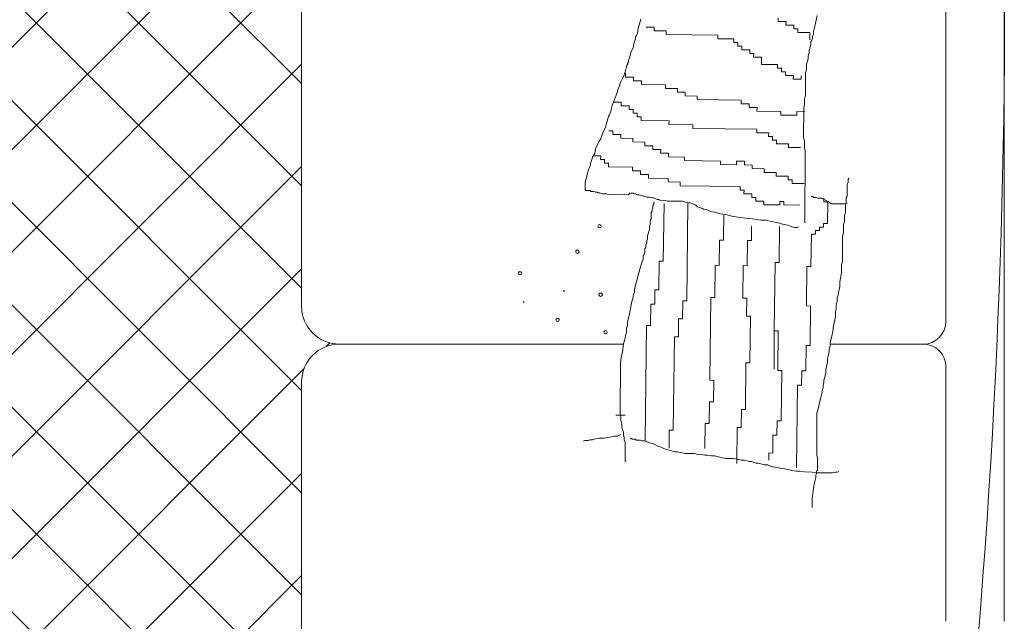
# Model space of a CAD drawing. Units: inches. Extents: x -466983 to 1020, y 324 to 318697.
# Tile 89 of 97: x 776 to 810, y 900 to 921. Entities that reach past the tile are written whole.
import ezdxf

# ---------------------------------------------------------------- set-up
doc = ezdxf.new("R2010")
doc.units = ezdxf.units.IN
doc.header["$MEASUREMENT"] = 0
doc.layers.add('A-FLOR-PATT', color=252, linetype='Continuous', lineweight=13)
doc.layers.add('A-FURN', color=8, linetype='Continuous', lineweight=18)

# ---------------------------------------------------------------- blocks, each defined once
blk = doc.blocks.new('L Shaped Sofa')
at = {"ltscale": 2}
for p, q in [((2356.696, 767.567), (2377.232, 767.567)), ((2377.232, 767.567), (2392.324, 767.567)), ((2429.959, 767.567), (2397.1, 767.567)), ((2394.712, 747.255), (2394.712, 765.179)), ((2388.636, 749.7), (2388.588, 749.809)), ((2388.634, 749.483), (2388.636, 749.7)), ((2388.683, 749.374), (2388.634, 749.483)), ((2388.682, 749.212), (2388.683, 749.374)), ((2404.345, 749.138), (2404.346, 749.301)), ((2404.346, 749.301), (2404.395, 749.355)), ((2404.395, 749.355), (2404.397, 749.626)), ((2404.397, 749.626), (2404.446, 749.68)), ((2404.446, 749.68), (2404.934, 749.678)), ((2404.934, 749.678), (2405.713, 749.457)), ((2405.713, 749.457), (2406.005, 749.347)), ((2406.005, 749.347), (2406.103, 749.347)), ((2406.103, 749.347), (2406.541, 749.182)), ((2388.729, 749.049), (2388.682, 749.212)), ((2388.776, 748.778), (2388.729, 749.049)), ((2388.775, 748.507), (2388.776, 748.778)), ((2404.193, 748.326), (2404.195, 748.597)), ((2404.195, 748.597), (2404.245, 748.759)), ((2404.245, 748.759), (2404.246, 748.868)), ((2404.246, 748.868), (2404.295, 748.922)), ((2404.295, 749.03), (2404.345, 749.138)), ((2404.295, 748.922), (2404.295, 749.03)), ((2406.349, 748.446), (2406.352, 748.698)), ((2406.352, 748.698), (2406.579, 748.695)), ((2406.541, 749.182), (2406.735, 749.073)), ((2406.579, 748.695), (2406.585, 749.199)), ((2406.735, 749.073), (2407.028, 749.017)), ((2407.028, 749.017), (2407.514, 748.798)), ((2407.514, 748.798), (2407.66, 748.689)), ((2407.66, 748.689), (2407.806, 748.634)), ((2407.806, 748.634), (2408.001, 748.579)), ((2388.822, 748.235), (2388.775, 748.507)), ((2388.917, 747.801), (2388.822, 748.235)), ((2404.136, 746.971), (2404.144, 748.218)), ((2404.144, 748.218), (2404.193, 748.326)), ((2405.873, 746.688), (2405.892, 748.199)), ((2405.892, 748.199), (2406.119, 748.197)), ((2406.119, 748.197), (2406.122, 748.449)), ((2406.122, 748.449), (2406.349, 748.446)), ((2408.001, 748.579), (2408.147, 748.524)), ((2408.147, 748.524), (2408.342, 748.415)), ((2408.157, 747.92), (2408.16, 748.172)), ((2408.342, 748.415), (2408.926, 748.249)), ((2408.926, 748.249), (2409.072, 748.194)), ((2409.072, 748.194), (2409.17, 748.14)), ((2409.17, 748.14), (2409.316, 748.085)), ((2409.316, 748.085), (2409.51, 748.03)), ((2409.51, 748.03), (2409.754, 747.974)), ((2409.754, 747.974), (2410.63, 747.645)), ((2388.916, 747.638), (2388.917, 747.801)), ((2389.012, 747.421), (2388.916, 747.638)), ((2389.304, 747.311), (2389.5, 747.365)), ((2389.5, 747.365), (2389.695, 747.364)), ((2389.695, 747.364), (2389.89, 747.417)), ((2389.89, 747.417), (2390.086, 747.416)), ((2390.086, 747.416), (2390.33, 747.469)), ((2390.234, 747.741), (2390.23, 747.144)), ((2390.33, 747.469), (2393.55, 747.454)), ((2393.55, 747.454), (2393.843, 747.398)), ((2393.843, 747.398), (2394.33, 747.288)), ((2407.688, 746.666), (2407.697, 747.422)), ((2407.697, 747.422), (2407.924, 747.419)), ((2407.924, 747.419), (2407.93, 747.923)), ((2407.93, 747.923), (2408.157, 747.92)), ((2409.733, 746.893), (2409.739, 747.397)), ((2409.739, 747.397), (2409.966, 747.394)), ((2409.966, 747.394), (2409.972, 747.898)), ((2410.63, 747.645), (2410.825, 747.59)), ((2410.825, 747.59), (2411.02, 747.48)), ((2411.02, 747.48), (2411.117, 747.48)), ((2411.117, 747.48), (2411.263, 747.425)), ((2411.263, 747.425), (2411.458, 747.316)), ((2387.302, 747.104), (2387.351, 747.158)), ((2387.351, 747.158), (2388.523, 747.152)), ((2388.523, 747.152), (2388.669, 747.206)), ((2388.669, 747.206), (2388.816, 747.205)), ((2388.715, 746.718), (2388.764, 746.772)), ((2388.764, 746.772), (2388.765, 746.826)), ((2388.816, 747.205), (2388.962, 747.259)), ((2388.962, 747.259), (2389.158, 747.258)), ((2389.158, 747.258), (2389.304, 747.311)), ((2394.33, 747.288), (2394.574, 747.287)), ((2394.574, 747.287), (2394.818, 747.231)), ((2394.818, 747.231), (2395.013, 747.176)), ((2395.013, 747.176), (2395.256, 747.121)), ((2395.256, 747.121), (2395.451, 747.066)), ((2395.451, 747.066), (2395.695, 747.064)), ((2395.695, 747.064), (2395.89, 747.009)), ((2395.89, 747.009), (2396.085, 747.008)), ((2396.085, 747.008), (2396.28, 746.953)), ((2396.28, 746.953), (2396.524, 746.898)), ((2396.524, 746.898), (2397.401, 746.731)), ((2397.401, 746.731), (2397.596, 746.676)), ((2404.233, 746.862), (2404.136, 746.971)), ((2404.232, 746.645), (2404.233, 746.862)), ((2409.503, 746.644), (2409.506, 746.896)), ((2409.506, 746.896), (2409.733, 746.893)), ((2411.458, 747.316), (2411.701, 747.206)), ((2411.544, 746.619), (2411.55, 747.123)), ((2411.55, 747.123), (2411.777, 747.12)), ((2411.701, 747.206), (2411.896, 747.151)), ((2411.896, 747.151), (2412.14, 747.096)), ((2412.14, 747.096), (2412.286, 747.041)), ((2412.286, 747.041), (2412.383, 746.986)), ((2412.383, 746.986), (2412.481, 746.986)), ((2412.481, 746.986), (2412.529, 746.931)), ((2412.529, 746.931), (2412.627, 746.931)), ((2412.627, 746.931), (2412.773, 746.876)), ((2412.773, 746.876), (2413.162, 746.766)), ((2413.162, 746.766), (2413.406, 746.656)), ((2388.614, 746.068), (2388.663, 746.176)), ((2388.663, 746.176), (2388.665, 746.447)), ((2388.665, 746.447), (2388.714, 746.501)), ((2388.714, 746.501), (2388.715, 746.718)), ((2397.596, 746.676), (2397.839, 746.621)), ((2397.839, 746.621), (2397.985, 746.566)), ((2397.985, 746.566), (2398.181, 746.565)), ((2398.181, 746.565), (2398.57, 746.455)), ((2398.57, 746.455), (2398.814, 746.399)), ((2398.814, 746.399), (2399.204, 746.289)), ((2399.204, 746.289), (2399.447, 746.234)), ((2399.447, 746.234), (2399.593, 746.179)), ((2399.593, 746.179), (2399.788, 746.123)), ((2399.788, 746.123), (2400.08, 746.014)), ((2403.983, 745.779), (2404.132, 746.266)), ((2404.132, 746.266), (2404.133, 746.374)), ((2404.133, 746.374), (2404.182, 746.482)), ((2404.182, 746.482), (2404.183, 746.591)), ((2404.183, 746.591), (2404.232, 746.645)), ((2405.407, 745.686), (2405.414, 746.19)), ((2405.414, 746.19), (2405.64, 746.187)), ((2405.64, 746.187), (2405.647, 746.691)), ((2405.647, 746.691), (2405.873, 746.688)), ((2407.452, 745.913), (2407.461, 746.669)), ((2407.461, 746.669), (2407.688, 746.666)), ((2408.795, 744.385), (2408.816, 746.148)), ((2408.816, 746.148), (2409.043, 746.145)), ((2409.043, 746.145), (2409.046, 746.397)), ((2409.046, 746.397), (2409.273, 746.394)), ((2409.273, 746.394), (2409.276, 746.646)), ((2409.276, 746.646), (2409.503, 746.644)), ((2411.066, 744.609), (2411.084, 746.12)), ((2411.084, 746.12), (2411.311, 746.118)), ((2411.311, 746.118), (2411.317, 746.621)), ((2411.317, 746.621), (2411.544, 746.619)), ((2413.406, 746.656), (2413.649, 746.601)), ((2413.649, 746.601), (2413.844, 746.545)), ((2413.844, 746.545), (2413.99, 746.491)), ((2413.99, 746.491), (2414.088, 746.49)), ((2414.088, 746.49), (2414.185, 746.435)), ((2414.185, 746.435), (2414.331, 746.381)), ((2414.331, 746.381), (2414.624, 746.325)), ((2414.624, 746.325), (2415.208, 746.16)), ((2388.414, 745.364), (2388.514, 745.688)), ((2388.514, 745.688), (2388.563, 745.797)), ((2388.563, 745.797), (2388.613, 745.959)), ((2388.613, 745.959), (2388.614, 746.068)), ((2388.622, 745.891), (2395.88, 745.802)), ((2395.88, 745.802), (2395.877, 745.55)), ((2395.877, 745.55), (2397.238, 745.534)), ((2397.238, 745.534), (2397.235, 745.282)), ((2400.08, 746.014), (2400.276, 746.013)), ((2400.276, 746.013), (2400.373, 745.958)), ((2400.373, 745.958), (2400.519, 745.903)), ((2400.519, 745.903), (2400.714, 745.902)), ((2400.714, 745.902), (2400.811, 745.848)), ((2400.811, 745.848), (2400.958, 745.847)), ((2400.958, 745.847), (2401.104, 745.792)), ((2401.104, 745.792), (2401.25, 745.791)), ((2401.25, 745.791), (2401.347, 745.737)), ((2401.347, 745.737), (2401.543, 745.736)), ((2401.543, 745.736), (2401.932, 745.625)), ((2401.932, 745.625), (2402.127, 745.625)), ((2402.127, 745.625), (2402.273, 745.57)), ((2402.273, 745.57), (2402.517, 745.569)), ((2402.517, 745.569), (2402.615, 745.514)), ((2402.615, 745.514), (2403.005, 745.512)), ((2403.005, 745.512), (2403.102, 745.457)), ((2403.932, 745.453), (2403.982, 745.616)), ((2403.982, 745.616), (2403.983, 745.779)), ((2405.165, 744.429), (2405.181, 745.689)), ((2405.181, 745.689), (2405.407, 745.686)), ((2407.219, 745.412), (2407.225, 745.916)), ((2407.225, 745.916), (2407.452, 745.913)), ((2414.705, 745.32), (2414.711, 745.824)), ((2388.117, 744.66), (2388.216, 744.877)), ((2388.216, 744.877), (2388.266, 745.039)), ((2388.266, 745.039), (2388.414, 745.364)), ((2397.235, 745.282), (2398.143, 745.271)), ((2398.143, 745.271), (2398.139, 745.019)), ((2398.139, 745.019), (2399.954, 744.997)), ((2399.954, 744.997), (2399.951, 744.745)), ((2403.102, 745.457), (2403.2, 745.457)), ((2403.2, 745.457), (2403.297, 745.402)), ((2403.297, 745.402), (2403.444, 745.402)), ((2403.444, 745.402), (2403.541, 745.347)), ((2403.541, 745.347), (2403.687, 745.346)), ((2403.78, 744.587), (2403.782, 744.966)), ((2403.782, 744.966), (2403.832, 745.02)), ((2403.832, 745.129), (2403.931, 745.345)), ((2403.832, 745.02), (2403.832, 745.129)), ((2403.931, 745.345), (2403.932, 745.453)), ((2406.753, 744.41), (2406.759, 744.914)), ((2406.759, 744.914), (2406.986, 744.911)), ((2406.986, 744.911), (2406.992, 745.415)), ((2406.992, 745.415), (2407.219, 745.412)), ((2414.469, 744.567), (2414.478, 745.323)), ((2414.478, 745.323), (2414.705, 745.32)), ((2387.918, 744.011), (2388.117, 744.66)), ((2388.149, 744.385), (2389.284, 744.371)), ((2389.284, 744.371), (2389.281, 744.119)), ((2399.951, 744.745), (2403.58, 744.7)), ((2403.725, 743.557), (2403.731, 744.478)), ((2403.731, 744.478), (2403.78, 744.587)), ((2404.929, 743.676), (2404.938, 744.432)), ((2404.938, 744.432), (2405.165, 744.429)), ((2406.514, 743.405), (2406.526, 744.412)), ((2406.526, 744.412), (2406.753, 744.41)), ((2408.549, 742.876), (2408.568, 744.388)), ((2408.568, 744.388), (2408.795, 744.385)), ((2410.83, 743.856), (2410.839, 744.612)), ((2410.839, 744.612), (2411.066, 744.609)), ((2414.202, 741.295), (2414.242, 744.57)), ((2414.242, 744.57), (2414.469, 744.567)), ((2387.866, 743.523), (2387.867, 743.685)), ((2387.867, 743.685), (2387.917, 743.848)), ((2387.917, 743.848), (2387.918, 744.011)), ((2389.281, 744.119), (2395.178, 744.047)), ((2395.178, 744.047), (2395.175, 743.795)), ((2395.175, 743.795), (2396.309, 743.781)), ((2396.309, 743.781), (2396.306, 743.53)), ((2404.656, 739.9), (2404.702, 743.679)), ((2404.702, 743.679), (2404.929, 743.676)), ((2410.597, 743.355), (2410.603, 743.859)), ((2410.603, 743.859), (2410.83, 743.856)), ((2387.813, 742.764), (2387.816, 743.36)), ((2387.816, 743.36), (2387.866, 743.523)), ((2396.306, 743.53), (2397.44, 743.516)), ((2397.44, 743.516), (2397.437, 743.264)), ((2397.437, 743.264), (2403.562, 743.189)), ((2403.575, 742.907), (2403.624, 743.069)), ((2403.624, 743.069), (2403.625, 743.232)), ((2403.625, 743.232), (2403.725, 743.557)), ((2406.259, 741.14), (2406.287, 743.408)), ((2406.287, 743.408), (2406.514, 743.405)), ((2410.361, 742.602), (2410.37, 743.358)), ((2410.37, 743.358), (2410.597, 743.355)), ((2387.761, 742.331), (2387.763, 742.656)), ((2387.763, 742.656), (2387.813, 742.764)), ((2403.278, 742.312), (2403.328, 742.474)), ((2403.328, 742.474), (2403.378, 742.583)), ((2403.378, 742.583), (2403.476, 742.69)), ((2403.476, 742.69), (2403.575, 742.907)), ((2408.273, 738.848), (2408.322, 742.879)), ((2408.322, 742.879), (2408.549, 742.876)), ((2410.1, 739.834), (2410.134, 742.605)), ((2410.134, 742.605), (2410.361, 742.602)), ((2387.66, 741.735), (2387.71, 741.951)), ((2387.71, 741.951), (2387.711, 742.114)), ((2387.711, 742.114), (2387.761, 742.331)), ((2388.122, 742.118), (2389.71, 742.098)), ((2389.71, 742.098), (2389.706, 741.847)), ((2389.706, 741.847), (2391.067, 741.83)), ((2391.067, 741.83), (2391.064, 741.578)), ((2392.425, 741.561), (2392.429, 741.813)), ((2392.429, 741.813), (2397.646, 741.75)), ((2403.029, 741.5), (2403.08, 741.771)), ((2403.08, 741.771), (2403.179, 741.987)), ((2403.179, 741.987), (2403.229, 742.204)), ((2403.229, 742.204), (2403.278, 742.312)), ((2387.558, 741.084), (2387.659, 741.518)), ((2387.659, 741.518), (2387.66, 741.735)), ((2391.064, 741.578), (2392.425, 741.561)), ((2397.646, 741.75), (2397.643, 741.498)), ((2397.643, 741.498), (2399.684, 741.473)), ((2399.684, 741.473), (2399.681, 741.221)), ((2399.681, 741.221), (2401.269, 741.201)), ((2401.269, 741.201), (2401.266, 740.949)), ((2402.879, 740.796), (2402.93, 741.175)), ((2402.93, 741.175), (2403.029, 741.5)), ((2406.02, 740.135), (2406.033, 741.143)), ((2406.033, 741.143), (2406.259, 741.14)), ((2413.963, 740.29), (2413.975, 741.298)), ((2413.975, 741.298), (2414.202, 741.295)), ((2387.505, 740.326), (2387.508, 740.814)), ((2387.508, 740.814), (2387.558, 741.084)), ((2401.266, 740.949), (2401.72, 740.944)), ((2401.493, 740.947), (2402.854, 740.93)), ((2401.72, 740.944), (2401.493, 740.947)), ((2402.779, 740.417), (2402.879, 740.796)), ((2387.19, 740.114), (2389.458, 740.086)), ((2387.404, 739.838), (2387.454, 740.055)), ((2387.454, 740.055), (2387.505, 740.326)), ((2389.458, 740.086), (2389.455, 739.834)), ((2402.626, 739.387), (2402.728, 740.037)), ((2402.728, 740.037), (2402.779, 740.417)), ((2404.426, 739.651), (2404.429, 739.903)), ((2404.429, 739.903), (2404.656, 739.9)), ((2406.247, 740.133), (2406.02, 740.135)), ((2406.241, 739.629), (2406.247, 740.133)), ((2413.503, 739.792), (2413.506, 740.044)), ((2413.506, 740.044), (2413.733, 740.041)), ((2413.733, 740.041), (2413.736, 740.293)), ((2413.736, 740.293), (2413.963, 740.29)), ((2387.303, 739.296), (2387.403, 739.621)), ((2387.303, 739.188), (2387.303, 739.296)), ((2387.403, 739.621), (2387.404, 739.838)), ((2389.455, 739.834), (2390.589, 739.82)), ((2390.589, 739.82), (2390.586, 739.568)), ((2390.586, 739.568), (2393.535, 739.532)), ((2393.535, 739.532), (2393.532, 739.28)), ((2393.532, 739.28), (2396.481, 739.244)), ((2396.481, 739.244), (2396.484, 739.496)), ((2396.484, 739.496), (2397.618, 739.482)), ((2397.618, 739.482), (2397.621, 739.734)), ((2397.621, 739.734), (2399.663, 739.709)), ((2399.663, 739.709), (2399.66, 739.457)), ((2399.66, 739.457), (2401.247, 739.438)), ((2401.247, 739.438), (2401.244, 739.186)), ((2402.624, 739.116), (2402.626, 739.387)), ((2404.193, 739.15), (2404.199, 739.654)), ((2404.199, 739.654), (2404.426, 739.651)), ((2406.008, 739.128), (2406.014, 739.632)), ((2406.014, 739.632), (2406.241, 739.629)), ((2409.634, 738.832), (2409.64, 739.335)), ((2409.64, 739.335), (2409.867, 739.333)), ((2409.867, 739.333), (2409.873, 739.836)), ((2409.873, 739.836), (2410.1, 739.834)), ((2413.04, 739.042), (2413.043, 739.294)), ((2413.043, 739.294), (2413.27, 739.291)), ((2413.27, 739.291), (2413.276, 739.795)), ((2413.276, 739.795), (2413.503, 739.792)), ((2387.153, 738.592), (2387.202, 738.755)), ((2387.202, 738.755), (2387.203, 738.917)), ((2387.203, 738.917), (2387.253, 739.026)), ((2387.253, 739.026), (2387.303, 739.188)), ((2394.569, 739.178), (2394.569, 739.178)), ((2401.244, 739.186), (2402.152, 739.175)), ((2402.523, 738.574), (2402.624, 739.116)), ((2403.73, 738.4), (2403.736, 738.904)), ((2403.736, 738.904), (2403.963, 738.901)), ((2403.963, 738.901), (2403.966, 739.153)), ((2403.966, 739.153), (2404.193, 739.15)), ((2405.772, 738.375), (2405.781, 739.131)), ((2405.781, 739.131), (2406.008, 739.128)), ((2408.037, 738.095), (2408.046, 738.851)), ((2408.046, 738.851), (2408.273, 738.848)), ((2409.389, 737.323), (2409.407, 738.834)), ((2409.407, 738.834), (2409.634, 738.832)), ((2412.807, 738.541), (2412.813, 739.045)), ((2412.813, 739.045), (2413.04, 739.042)), ((2387.002, 737.942), (2387.101, 738.159)), ((2387.101, 738.159), (2387.103, 738.376)), ((2387.103, 738.376), (2387.153, 738.592)), ((2387.392, 738.096), (2387.846, 738.09)), ((2387.846, 738.09), (2387.843, 737.838)), ((2402.37, 737.491), (2402.522, 738.303)), ((2402.522, 738.303), (2402.523, 738.574)), ((2403.491, 737.395), (2403.503, 738.403)), ((2403.503, 738.403), (2403.73, 738.4)), ((2405.536, 737.622), (2405.545, 738.378)), ((2405.545, 738.378), (2405.772, 738.375)), ((2407.807, 737.846), (2407.81, 738.098)), ((2407.81, 738.098), (2408.037, 738.095)), ((2412.341, 737.539), (2412.353, 738.546)), ((2412.353, 738.546), (2412.807, 738.541)), ((2386.8, 736.859), (2387.002, 737.942)), ((2387.843, 737.838), (2388.977, 737.824)), ((2388.977, 737.824), (2388.974, 737.572)), ((2388.974, 737.572), (2389.881, 737.561)), ((2389.881, 737.561), (2389.878, 737.309)), ((2393.054, 737.271), (2393.057, 737.522)), ((2393.057, 737.522), (2395.552, 737.492)), ((2396.001, 737.746), (2393.136, 737.746)), ((2395.552, 737.492), (2395.555, 737.744)), ((2395.555, 737.744), (2399.865, 737.691)), ((2399.865, 737.691), (2399.862, 737.439)), ((2399.862, 737.439), (2402.13, 737.412)), ((2402.271, 737.22), (2402.37, 737.491)), ((2405.3, 736.869), (2405.309, 737.625)), ((2405.309, 737.625), (2405.536, 737.622)), ((2407.341, 736.844), (2407.35, 737.6)), ((2407.35, 737.6), (2407.577, 737.597)), ((2407.577, 737.597), (2407.58, 737.849)), ((2407.58, 737.849), (2407.807, 737.846)), ((2412.111, 737.29), (2412.114, 737.542)), ((2412.114, 737.542), (2412.341, 737.539)), ((2415.057, 737.002), (2415.063, 737.506)), ((2415.063, 737.506), (2415.29, 737.503)), ((2386.75, 736.642), (2386.8, 736.859)), ((2389.878, 737.309), (2393.054, 737.271)), ((2402.121, 736.679), (2402.22, 736.895)), ((2402.22, 736.895), (2402.271, 737.22)), ((2403.476, 736.135), (2403.488, 737.143)), ((2403.488, 737.143), (2403.715, 737.14)), ((2403.718, 737.392), (2403.491, 737.395)), ((2403.715, 737.14), (2403.718, 737.392)), ((2405.07, 736.62), (2405.073, 736.872)), ((2405.073, 736.872), (2405.3, 736.869)), ((2407.105, 736.091), (2407.114, 736.847)), ((2407.114, 736.847), (2407.341, 736.844)), ((2409.15, 736.318), (2409.162, 737.326)), ((2409.162, 737.326), (2409.389, 737.323)), ((2411.648, 736.539), (2411.654, 737.043)), ((2411.654, 737.043), (2411.881, 737.041)), ((2411.881, 737.041), (2411.884, 737.292)), ((2411.884, 737.292), (2412.111, 737.29)), ((2414.824, 736.501), (2414.83, 737.004)), ((2414.83, 737.004), (2415.057, 737.002)), ((2386.698, 736.101), (2386.7, 736.372)), ((2386.7, 736.372), (2386.75, 736.642)), ((2386.917, 736.338), (2392.134, 736.274)), ((2392.134, 736.274), (2392.131, 736.022)), ((2402.07, 736.299), (2402.071, 736.462)), ((2402.118, 736.191), (2402.07, 736.299)), ((2402.071, 736.462), (2402.121, 736.679)), ((2404.834, 735.867), (2404.843, 736.623)), ((2404.843, 736.623), (2405.07, 736.62)), ((2409.377, 736.315), (2409.15, 736.318)), ((2409.37, 735.811), (2409.377, 736.315)), ((2411.415, 736.038), (2411.421, 736.542)), ((2411.421, 736.542), (2411.648, 736.539)), ((2414.358, 735.499), (2414.367, 736.254)), ((2414.367, 736.254), (2414.594, 736.252)), ((2414.594, 736.252), (2414.597, 736.503)), ((2414.597, 736.503), (2414.824, 736.501)), ((2386.645, 735.342), (2386.648, 735.83)), ((2386.648, 735.83), (2386.698, 736.101)), ((2392.131, 736.022), (2393.038, 736.011)), ((2393.038, 736.011), (2393.035, 735.759)), ((2393.035, 735.759), (2394.623, 735.74)), ((2394.623, 735.74), (2394.62, 735.488)), ((2397.115, 735.457), (2397.118, 735.709)), ((2397.118, 735.709), (2399.613, 735.679)), ((2399.613, 735.679), (2399.61, 735.427)), ((2402.36, 735.81), (2406.898, 735.789)), ((2406.898, 735.789), (2407.094, 735.842)), ((2407.094, 735.842), (2407.533, 735.84)), ((2407.533, 735.84), (2407.728, 735.893)), ((2407.728, 735.893), (2409.582, 735.885)), ((2409.582, 735.885), (2409.875, 735.829)), ((2409.875, 735.829), (2410.168, 735.828)), ((2410.168, 735.828), (2410.411, 735.772)), ((2410.411, 735.772), (2411.826, 735.766)), ((2411.642, 736.036), (2411.415, 736.038)), ((2411.826, 735.766), (2412.021, 735.711)), ((2412.021, 735.711), (2412.363, 735.709)), ((2412.363, 735.709), (2412.558, 735.654)), ((2412.558, 735.654), (2412.704, 735.599)), ((2412.704, 735.599), (2412.899, 735.598)), ((2412.899, 735.598), (2413.094, 735.543)), ((2384.4, 735.352), (2384.986, 735.349)), ((2384.986, 735.349), (2385.766, 735.237)), ((2385.766, 735.237), (2386.058, 735.182)), ((2386.058, 735.182), (2386.302, 735.126)), ((2386.302, 735.126), (2386.448, 735.126)), ((2386.448, 735.126), (2386.546, 735.071)), ((2386.546, 735.071), (2386.692, 735.07)), ((2386.588, 734.095), (2386.595, 735.125)), ((2386.595, 735.125), (2386.645, 735.342)), ((2386.692, 735.07), (2386.74, 735.016)), ((2386.74, 735.016), (2387.57, 735.012)), ((2387.57, 735.012), (2387.717, 735.066)), ((2387.717, 735.066), (2390.352, 735.053)), ((2390.352, 735.053), (2390.546, 734.998)), ((2390.546, 734.998), (2391.277, 734.832)), ((2394.62, 735.488), (2397.115, 735.457)), ((2399.61, 735.427), (2401.652, 735.402)), ((2401.652, 735.402), (2401.649, 735.15)), ((2401.649, 735.15), (2401.876, 735.147)), ((2401.876, 735.147), (2401.873, 734.895)), ((2403.915, 734.773), (2403.917, 734.99)), ((2403.917, 734.99), (2403.966, 735.098)), ((2403.966, 735.098), (2403.967, 735.26)), ((2403.967, 735.26), (2404.016, 735.314)), ((2404.016, 735.314), (2404.017, 735.423)), ((2413.094, 735.543), (2413.24, 735.542)), ((2413.24, 735.542), (2413.63, 735.432)), ((2413.63, 735.432), (2413.776, 735.431)), ((2413.776, 735.431), (2413.873, 735.377)), ((2413.873, 735.377), (2414.019, 735.322)), ((2413.904, 735.504), (2414.358, 735.499)), ((2414.019, 735.322), (2414.117, 735.321)), ((2414.117, 735.321), (2414.263, 735.266)), ((2414.263, 735.266), (2414.458, 735.265)), ((2414.458, 735.265), (2414.653, 735.21)), ((2414.653, 735.21), (2415.14, 735.1)), ((2415.14, 735.1), (2415.433, 735.044)), ((2391.277, 734.832), (2391.667, 734.722)), ((2391.667, 734.722), (2391.813, 734.721)), ((2391.813, 734.721), (2391.959, 734.666)), ((2391.959, 734.666), (2392.106, 734.665)), ((2392.106, 734.665), (2392.301, 734.61)), ((2392.301, 734.61), (2392.447, 734.61)), ((2392.447, 734.61), (2392.642, 734.555)), ((2392.642, 734.555), (2392.886, 734.499)), ((2392.886, 734.499), (2393.081, 734.498)), ((2393.081, 734.498), (2393.568, 734.388)), ((2393.568, 734.388), (2393.812, 734.386)), ((2393.812, 734.386), (2394.056, 734.331)), ((2394.056, 734.331), (2394.25, 734.276)), ((2401.873, 734.895), (2402.099, 734.892)), ((2402.099, 734.892), (2402.096, 734.641)), ((2402.096, 734.641), (2402.323, 734.638)), ((2402.323, 734.638), (2402.32, 734.386)), ((2402.32, 734.386), (2403.681, 734.369)), ((2403.619, 734.232), (2403.717, 734.34)), ((2403.681, 734.369), (2403.684, 734.621)), ((2403.684, 734.621), (2403.911, 734.618)), ((2403.717, 734.34), (2403.915, 734.773)), ((2386.636, 733.878), (2386.588, 734.095)), ((2386.635, 733.769), (2386.636, 733.878)), ((2386.683, 733.661), (2386.635, 733.769)), ((2394.25, 734.276), (2394.397, 734.275)), ((2394.397, 734.275), (2394.592, 734.22)), ((2394.592, 734.22), (2394.787, 734.219)), ((2394.712, 728.35), (2394.712, 734.219)), ((2394.787, 734.219), (2394.982, 734.164)), ((2394.982, 734.164), (2395.225, 734.109)), ((2395.225, 734.109), (2395.518, 734.053)), ((2395.518, 734.053), (2395.859, 733.997)), ((2395.859, 733.997), (2396.444, 733.886)), ((2396.444, 733.886), (2396.737, 733.885)), ((2396.737, 733.885), (2396.98, 733.829)), ((2396.98, 733.829), (2397.176, 733.828)), ((2397.176, 733.828), (2397.419, 733.773)), ((2397.419, 733.773), (2397.614, 733.772)), ((2397.614, 733.772), (2397.809, 733.717)), ((2397.809, 733.717), (2398.053, 733.662)), ((2403.565, 733.31), (2403.57, 734.124)), ((2403.57, 734.124), (2403.619, 734.232)), ((2398.053, 733.662), (2398.345, 733.606)), ((2398.345, 733.606), (2398.638, 733.605)), ((2398.638, 733.605), (2399.223, 733.493)), ((2399.223, 733.493), (2399.711, 733.491)), ((2399.711, 733.491), (2399.906, 733.436)), ((2399.906, 733.436), (2401.516, 733.429)), ((2401.516, 733.429), (2401.76, 733.373)), ((2401.76, 733.373), (2402.248, 733.371)), ((2402.248, 733.371), (2402.442, 733.316)), ((2402.442, 733.316), (2402.833, 733.314)), ((2402.833, 733.314), (2403.028, 733.259)), ((2403.028, 733.259), (2403.467, 733.257)), ((2403.467, 733.257), (2403.613, 733.202)), ((2403.613, 733.148), (2403.565, 733.31)), ((2403.613, 733.202), (2403.954, 733.2)), ((2403.954, 733.2), (2404.052, 733.146)), ((2404.052, 733.146), (2404.784, 733.142)), ((2404.784, 733.142), (2404.93, 733.087)), ((2404.93, 733.087), (2405.125, 733.086)), ((2405.125, 733.086), (2405.173, 733.032)), ((2393.28, 726.917), (2377.232, 726.917)), ((2430.914, 726.917), (2396.145, 726.917)), ((2475.263, 723.229), (2377.232, 723.229))]:
    blk.add_line(p, q, dxfattribs=at)
for centre, radius, start, end in [((2392.324, 765.179), 2.388, 0, 90), ((2397.1, 765.179), 2.388, 90, 180), ((2397.375, 753.562), 0.0177, 90, 270), ((2397.375, 753.562), 0.0177, 270, 90), ((2399.184, 753.788), 0.106, 90, 270), ((2399.184, 753.788), 0.106, 270, 90), ((2396.244, 751.412), 0.106, 90, 270), ((2396.244, 751.412), 0.106, 270, 90), ((2398.074, 751.018), 0.0177, 90, 270), ((2398.074, 751.018), 0.0177, 270, 90), ((2400.541, 750.168), 0.106, 90, 270), ((2400.541, 750.168), 0.106, 270, 90), ((2397.827, 748.697), 0.106, 90, 270), ((2397.827, 748.697), 0.106, 270, 90), ((2402.147, 748.771), 0.106, 90, 270), ((2402.147, 748.771), 0.106, 270, 90), ((2395.463, 748.389), 0.106, 90, 270), ((2395.463, 748.389), 0.106, 270, 90), ((2393.28, 728.35), 1.433, 270, 0), ((2396.145, 728.35), 1.433, 180, 270), ((2416.36, 1205.029), 481.82, 262.88673, 276.63201)]:
    blk.add_arc(centre, radius, start, end, dxfattribs=at)

msp = doc.modelspace()

# ---------------------------------------------------------------- hatches: boundary and pattern name
at = {"layer": 'A-FLOR-PATT', "transparency": 33554572}
h = msp.add_hatch(dxfattribs=at)
h.set_pattern_fill('ANSI37', color=256, scale=30)
h.set_pattern_definition([(45, (-1212.4137, -290.035), (-2.6516504, 2.6516504), []), (135, (-1212.4137, -290.035), (-2.6516504, -2.6516504), [])])
h.paths.add_polyline_path([(901.806, 1075.938), (900.614, 1075.938), (900.614, 1065.386), (899.391, 1065.386), (898.091, 1065.386), (892.836, 1058.71, -0.258377), (892.188, 1058.351), (879.985, 1058.351, -0.20177), (879.438, 1058.581), (874.081, 1065.386), (872.781, 1065.386), (871.558, 1065.386), (871.558, 1075.938), (813.806, 1075.938), (813.806, 1044.792), (832.395, 1044.792, -0.394795), (848.66, 1028.536), (848.66, 1009.938), (901.806, 1009.938), (901.806, 1015.938), (901.306, 1015.938), (871.306, 1015.938), (871.306, 1017.25), (871.334, 1017.25, -0.401453), (901.306, 1045.938), (901.806, 1045.938)])
edge = h.paths.add_edge_path(flags=16)
edge.add_line((847.773, 1068.949), (847.773, 1073.709))
edge.add_arc((849.227, 1073.709), 1.454, 90, 180, ccw=False)
edge.add_line((849.227, 1075.163), (864.492, 1075.163))
edge.add_arc((864.492, 1073.709), 1.454, 0, 90, ccw=False)
edge.add_line((865.946, 1073.709), (865.946, 1069.004))
edge.add_arc((832.645, 1068.976), 33.301, -20.6123, 0.0472, ccw=False)
edge.add_ellipse((856.859, 1058.48), major_axis=(0, 10.213), ratio=0.685919, start_angle=100.0088, end_angle=259.9912, ccw=False)
edge.add_arc((881.074, 1068.976), 33.301, 180.0472, 200.6123, ccw=False)
h.paths.add_polyline_path([(853.146, 1066.482), (853.146, 1066.453), (853.146, 1066.453, 0.433107), (852.917, 1066.685), (852.917, 1066.453), (853.146, 1066.453), (853.146, 1066.482), (853.088, 1066.612, 0.697939), (852.7, 1066.453), (852.7, 1066.453), (852.7, 1066.482), (852.917, 1067.001), (852.917, 1066.685, -0.396254)], flags=0)
h.paths.add_polyline_path([(861.019, 1066.482), (861.019, 1066.453), (861.019, 1066.453, 0.416404), (860.802, 1066.685), (860.802, 1066.453), (861.019, 1066.453), (861.019, 1066.482), (860.967, 1066.605, 0.713344), (860.573, 1066.453), (860.573, 1066.453), (860.573, 1066.482), (860.802, 1067.001), (860.802, 1066.685, -0.379973)], flags=0)
edge = h.paths.add_edge_path(flags=0)
edge.add_spline(control_points=[(861.13, 1065.785), (861.466, 1065.248), (861.613, 1065.016), (861.983, 1064.374), (862.192, 1063.944), (862.561, 1063.039), (862.721, 1062.563), (862.987, 1061.578), (863.092, 1061.069), (863.245, 1060.031), (863.293, 1059.503), (863.329, 1058.441), (863.318, 1057.908), (863.237, 1056.852), (863.166, 1056.329), (862.97, 1055.308), (862.843, 1054.81), (862.537, 1053.852), (862.357, 1053.393), (861.951, 1052.525), (861.725, 1052.117), (861.233, 1051.362), (860.967, 1051.016), (860.405, 1050.395), (860.108, 1050.12), (859.494, 1049.646), (859.176, 1049.448), (858.528, 1049.13), (858.197, 1049.011), (857.531, 1048.852), (857.196, 1048.812), (856.525, 1048.812), (856.189, 1048.852), (855.524, 1049.01), (855.193, 1049.129), (854.545, 1049.447), (854.227, 1049.645), (853.612, 1050.118), (853.316, 1050.393), (852.753, 1051.014), (852.487, 1051.36), (851.995, 1052.114), (851.769, 1052.523), (851.363, 1053.39), (851.183, 1053.85), (850.877, 1054.807), (850.75, 1055.305), (850.553, 1056.326), (850.483, 1056.849), (850.401, 1057.905), (850.39, 1058.438), (850.426, 1059.5), (850.473, 1060.028), (850.626, 1061.066), (850.732, 1061.575), (850.997, 1062.561), (851.157, 1063.036), (851.525, 1063.942), (851.734, 1064.371), (852.106, 1065.016), (852.254, 1065.25), (852.608, 1065.733)], knot_values=[3.915332, 3.915332, 3.915332, 3.915332, 4.013468, 4.013468, 4.175532, 4.175532, 4.337596, 4.337596, 4.49966, 4.49966, 4.661724, 4.661724, 4.823788, 4.823788, 4.985852, 4.985852, 5.147916, 5.147916, 5.30998, 5.30998, 5.472044, 5.472044, 5.634109, 5.634109, 5.796173, 5.796173, 5.958237, 5.958237, 6.120301, 6.120301, 6.282365, 6.282365, 6.444429, 6.444429, 6.606493, 6.606493, 6.768557, 6.768557, 6.930621, 6.930621, 7.092685, 7.092685, 7.254749, 7.254749, 7.416813, 7.416813, 7.578878, 7.578878, 7.740942, 7.740942, 7.903006, 7.903006, 8.06507, 8.06507, 8.227134, 8.227134, 8.389198, 8.389198, 8.551262, 8.551262, 8.65037, 8.65037, 8.65037, 8.65037], degree=3, periodic=0)
edge.add_line((852.642, 1065.785), (861.13, 1065.785))
edge = h.paths.add_edge_path(flags=0)
edge.add_ellipse((856.85, 1057.743), major_axis=(0, 7.792), ratio=0.687861, start_angle=0, end_angle=360)
h.paths.add_polyline_path([(848.863, 1069.389), (848.863, 1073.96, -0.414214), (849.954, 1075.051), (863.765, 1075.051, -0.414214), (864.856, 1073.96), (864.856, 1069.389, -0.388936), (864.524, 1069.027, -0.043561), (849.195, 1069.027, -0.388936)], flags=0)
h.paths.add_polyline_path([(853.101, 1068.112, -1), (852.677, 1068.112, -1)], flags=0)
edge = h.paths.add_edge_path(flags=0)
edge.add_ellipse((856.859, 1057.338), major_axis=(0, 2.207), ratio=0.657164, start_angle=0, end_angle=360)
h.paths.add_polyline_path([(861.041, 1068.112, -1), (860.618, 1068.112, -1)], flags=0)
edge = h.paths.add_edge_path()
edge.add_line((573.954, 1057.341), (573.954, 1075.938))
edge.add_line((573.954, 1075.938), (558.731, 1075.938))
edge.add_line((558.731, 1075.938), (558.731, 1065.386))
edge.add_line((558.731, 1065.386), (557.507, 1065.386))
edge.add_line((557.507, 1065.386), (556.207, 1065.386))
edge.add_line((556.207, 1065.386), (550.952, 1058.71))
edge.add_arc((550.304, 1059.116), 0.765, 270, 327.9483, ccw=False)
edge.add_line((550.304, 1058.351), (538.101, 1058.351))
edge.add_arc((538.101, 1059.116), 0.765, 224.3704, 270, ccw=False)
edge.add_line((537.555, 1058.581), (532.198, 1065.386))
edge.add_line((532.198, 1065.386), (530.898, 1065.386))
edge.add_line((530.898, 1065.386), (529.674, 1065.386))
edge.add_line((529.674, 1065.386), (529.674, 1075.938))
edge.add_line((529.674, 1075.938), (520.806, 1075.938))
edge.add_line((520.806, 1075.938), (520.806, 1045.938))
edge.add_line((520.806, 1045.938), (521.306, 1045.938))
edge.add_arc((521.306, 1015.938), 30, 2.5075, 90, ccw=False)
edge.add_line((551.277, 1017.25), (551.306, 1017.25))
edge.add_line((551.306, 1017.25), (551.306, 1015.938))
edge.add_line((551.306, 1015.938), (520.806, 1015.938))
edge.add_line((520.806, 1015.938), (520.806, 1009.938))
edge.add_line((520.806, 1009.938), (559.191, 1010.402))
edge.add_arc((559.191, 1011.856), 1.454, 180, 270, ccw=False)
edge.add_line((557.737, 1011.856), (557.737, 1016.561))
edge.add_arc((591.039, 1016.589), 33.301, 159.3877, 180.0472, ccw=False)
edge.add_ellipse((566.824, 1027.085), major_axis=(0, 10.213), ratio=0.685919, start_angle=280.0088, end_angle=439.9912, ccw=False)
edge.add_arc((542.609, 1016.589), 33.301, 0.0472, 20.6123, ccw=False)
edge.add_line((575.91, 1016.616), (575.91, 1011.856))
edge.add_arc((574.456, 1011.856), 1.454, -90, 0, ccw=False)
edge.add_line((574.456, 1010.402), (608.806, 1009.938))
edge.add_line((608.806, 1009.938), (608.806, 1041.086))
edge.add_line((608.806, 1041.086), (590.218, 1041.086))
edge.add_arc((590.775, 1057.907), 16.831, 181.9277, 268.1032, ccw=False)
edge = h.paths.add_edge_path()
edge.add_ellipse((494.244, 583.62), major_axis=(0, 10.213), ratio=0.685919, start_angle=280.0088, end_angle=439.9912, ccw=False)
edge.add_arc((470.03, 573.124), 33.301, 0.0472, 20.6123, ccw=False)
edge.add_line((503.331, 573.152), (503.331, 568.392))
edge.add_arc((501.877, 568.392), 1.454, -90, 0, ccw=False)
edge.add_line((501.877, 566.938), (539.806, 566.938))
edge.add_line((539.806, 566.938), (539.806, 572.938))
edge.add_line((539.806, 572.938), (539.306, 572.938))
edge.add_line((539.306, 572.938), (509.306, 572.938))
edge.add_line((509.306, 572.938), (509.306, 574.25))
edge.add_line((509.306, 574.25), (509.334, 574.25))
edge.add_arc((539.306, 572.938), 30, 90, 177.4925, ccw=False)
edge.add_line((539.306, 602.938), (539.806, 602.938))
edge.add_line((539.806, 602.938), (539.806, 626.938))
edge.add_line((539.806, 626.938), (531.772, 626.938))
edge.add_line((531.772, 626.938), (531.772, 616.386))
edge.add_line((531.772, 616.386), (530.548, 616.386))
edge.add_line((530.548, 616.386), (529.249, 616.386))
edge.add_line((529.249, 616.386), (523.711, 609.351))
edge.add_line((523.711, 609.351), (510.777, 609.351))
edge.add_line((510.777, 609.351), (505.239, 616.386))
edge.add_line((505.239, 616.386), (503.939, 616.386))
edge.add_line((503.939, 616.386), (502.715, 616.386))
edge.add_line((502.715, 616.386), (502.715, 626.938))
edge.add_line((502.715, 626.938), (481.698, 626.938))
edge.add_line((481.698, 626.938), (481.698, 610.995))
edge.add_arc((467.27, 611.473), 14.436, 271.9277, 358.1032, ccw=False)
edge.add_line((467.756, 597.045), (451.806, 597.045))
edge.add_line((451.806, 597.045), (451.806, 584.404))
edge.add_line((451.806, 584.404), (451.806, 566.938))
edge.add_line((451.806, 566.938), (486.612, 566.938))
edge.add_arc((486.612, 568.392), 1.454, 180, 270, ccw=False)
edge.add_line((485.158, 568.392), (485.158, 573.097))
edge.add_arc((518.459, 573.124), 33.301, 159.3877, 180.0472, ccw=False)
h.paths.add_polyline_path([(836.261, 1020.733), (879.89, 1020.733), (879.89, 1039.39), (836.261, 1039.39)], flags=25)
h.paths.add_polyline_path([(549.985, 1036.749), (593.614, 1036.749), (593.614, 1055.407), (549.985, 1055.407)], flags=24)
h.paths.add_polyline_path([(475.123, 595.596), (518.752, 595.596), (518.752, 614.253), (475.123, 614.253)], flags=24)
h = msp.add_hatch(dxfattribs=at)
h.set_pattern_fill('ANSI37', color=256, scale=20)
h.set_pattern_definition([(45, (-1212.4137, -290.035), (-1.767767, 1.767767), []), (135, (-1212.4137, -290.035), (-1.767767, -1.767767), [])])
h.paths.add_polyline_path([(809.806, 870.938), (809.806, 888.152), (806.998, 888.152), (802.662, 888.152), (789.383, 888.152), (786.285, 888.152, -0.414214), (785.499, 888.937), (785.499, 900.196), (785.499, 908.47, -0.414214), (786.808, 909.779, -0.414214), (785.499, 911.088), (785.499, 929.101, -0.414214), (786.808, 930.411, -0.414214), (785.499, 931.72), (785.499, 931.904, -0.414214), (784.19, 930.595), (766.722, 930.595, -0.412359), (765.413, 931.896, -0.413741), (764.115, 930.578), (744.578, 930.422, -0.416556), (743.786, 931.207), (743.786, 933.515), (742.215, 933.515), (742.215, 952.024, -0.001344), (743.786, 952.2), (743.786, 953.938), (678.592, 953.938), (678.592, 951.131), (678.592, 946.794), (678.592, 933.515), (678.592, 930.417, -0.414214), (677.806, 929.631), (666.548, 929.631), (658.274, 929.631, -0.414214), (656.965, 930.94, -0.414214), (655.656, 929.631), (637.642, 929.631, -0.414214), (636.333, 930.94, -0.414214), (635.024, 929.631), (634.839, 929.631, -0.414214), (636.149, 928.322), (636.149, 910.854, -0.412359), (634.848, 909.545, -0.413741), (636.165, 908.247), (636.321, 888.71, -0.416556), (635.536, 887.918), (633.228, 887.918), (633.228, 886.347), (614.719, 886.347, -0.001344), (614.544, 887.918), (612.806, 887.918), (612.806, 834.938), (612.806, 752.938), (612.806, 748.938), (612.806, 697.938), (654.806, 697.938), (654.806, 701.938), (715.806, 701.938), (715.806, 737.435), (774.292, 737.435), (774.292, 795.938), (809.806, 795.938)])
h.paths.add_polyline_path([(679.276, 849.576, 0.102523), (682.148, 849.261, -0.080461), (694.543, 849.773, -0.283899), (694.482, 849.008, 0.136605), (694.407, 848.81, -0.030441), (694.543, 846.893), (694.543, 842.62), (694.543, 838.347, -0.028219), (694.425, 836.568), (694.425, 836.568, 0.196187), (694.446, 836.271, -0.302897), (694.543, 835.467, -0.080461), (682.148, 835.979, 0.102523), (679.276, 835.664, -0.58611), (678.646, 836.017), (678.646, 849.223, -0.58611)], flags=16)
h.paths.add_polyline_path([(679.517, 848.651, 0.699597), (679.476, 848.634, 1.20716), (679.194, 848.742, 0.010621)], flags=0)
h.paths.add_polyline_path([(679.492, 836.561, -0.013798), (679.918, 836.659, -0.071703), (682.853, 837.143, -0.165743), (682.166, 839.101), (682.166, 842.609), (682.166, 846.06, -0.240616), (683.473, 848.677, -0.068263), (693.929, 849.008), (693.788, 848.708), (693.788, 849.023, 0.067332), (683.473, 848.677, 0.240616), (682.166, 846.06), (682.166, 842.609), (682.166, 839.101, 0.23459), (683.461, 836.551, 0.068093), (693.788, 836.195), (693.788, 836.51), (693.93, 836.21, -0.077215), (682.242, 836.782, 0.086627), (679.528, 836.57, -0.628402), (679.503, 836.573), (679.503, 836.607, 0.910458)], flags=0)
h.paths.add_polyline_path([(679.476, 848.636), (679.207, 848.647), (679.207, 836.572, 0.913566), (679.365, 836.586), (679.476, 836.582)], flags=0)
h.paths.add_polyline_path([(679.276, 829.86, 0.102523), (682.148, 829.546, -0.080461), (694.543, 830.057, -0.283899), (694.482, 829.293, 0.136605), (694.407, 829.095, -0.030441), (694.543, 827.178), (694.543, 822.904), (694.543, 818.631, -0.028219), (694.425, 816.853), (694.425, 816.853, 0.196187), (694.446, 816.556, -0.302897), (694.543, 815.752, -0.080461), (682.148, 816.263, 0.102523), (679.276, 815.949, -0.58611), (678.646, 816.302), (678.646, 829.507, -0.58611)], flags=16)
h.paths.add_polyline_path([(679.517, 828.936, 0.699597), (679.476, 828.919, 1.20716), (679.194, 829.027, 0.010621)], flags=0)
h.paths.add_polyline_path([(679.492, 816.846, -0.013798), (679.918, 816.944, -0.071703), (682.853, 817.428, -0.165743), (682.166, 819.385), (682.166, 822.894), (682.166, 826.345, -0.240616), (683.473, 828.961, -0.068263), (693.929, 829.293), (693.788, 828.993), (693.788, 829.308, 0.067332), (683.473, 828.961, 0.240616), (682.166, 826.345), (682.166, 822.894), (682.166, 819.385, 0.23459), (683.461, 816.836, 0.068093), (693.788, 816.48), (693.788, 816.795), (693.93, 816.495, -0.077215), (682.242, 817.066, 0.086627), (679.528, 816.855, -0.628402), (679.503, 816.858), (679.503, 816.892, 0.910458)], flags=0)
h.paths.add_polyline_path([(679.476, 828.921), (679.207, 828.932), (679.207, 816.857, 0.913566), (679.365, 816.871), (679.476, 816.867)], flags=0)
h.paths.add_polyline_path([(679.276, 810.145, 0.102523), (682.148, 809.83, -0.080461), (694.543, 810.342, -0.3023), (694.447, 809.539, 0.10023), (694.406, 809.388, -0.03057), (694.543, 807.462), (694.543, 803.189), (694.543, 798.916, -0.03057), (694.406, 796.991, 0.10023), (694.447, 796.839, -0.3023), (694.543, 796.036, -0.080461), (682.148, 796.548, 0.102523), (679.276, 796.233, -0.58611), (678.646, 796.586), (678.646, 809.792, -0.58611)], flags=16)
h.paths.add_polyline_path([(679.517, 809.242, 0.699597), (679.476, 809.224, 1.20716), (679.194, 809.332, 0.010621)], flags=0)
h.paths.add_polyline_path([(679.492, 797.151, -0.013798), (679.918, 797.25, -0.071703), (682.853, 797.734, -0.165743), (682.166, 799.691), (682.166, 803.2), (682.166, 806.65, -0.239349), (683.461, 809.258, -0.072465), (694.447, 809.541, 0.197932), (694.425, 809.241), (693.788, 809.299), (693.788, 809.614, 0.068093), (683.461, 809.258, 0.239349), (682.166, 806.65), (682.166, 803.2), (682.166, 799.691, 0.235854), (683.473, 797.132, 0.067332), (693.788, 796.786), (693.788, 797.101), (694.425, 797.159, 0.197932), (694.447, 796.859, -0.080419), (682.156, 797.379, 0.083867), (679.528, 797.16, -0.628402), (679.503, 797.164), (679.503, 797.197, 0.910458)], flags=0)
h.paths.add_polyline_path([(679.207, 809.237), (679.207, 797.162, 0.913566), (679.365, 797.176), (679.476, 797.173), (679.476, 809.227)], flags=0)
h.paths.add_polyline_path([(695.364, 853.299), (728.223, 853.299), (728.223, 771.152), (695.364, 771.152)], flags=16)
h.paths.add_polyline_path([(696.021, 852.642), (727.566, 852.642), (727.566, 771.809), (696.021, 771.809)], flags=0)
h.paths.add_polyline_path([(679.276, 788.787, 0.102523), (682.148, 788.472, -0.080461), (694.543, 788.984, -0.3023), (694.447, 788.181, 0.10023), (694.406, 788.03, -0.03057), (694.543, 786.104), (694.543, 781.831), (694.543, 777.558, -0.03057), (694.406, 775.632, 0.10023), (694.447, 775.481, -0.3023), (694.543, 774.678, -0.080461), (682.148, 775.19, 0.102523), (679.276, 774.875, -0.58611), (678.646, 775.228), (678.646, 788.434, -0.58611)], flags=16)
h.paths.add_polyline_path([(679.517, 787.883, 0.699597), (679.476, 787.866, 1.20716), (679.194, 787.974, 0.010621)], flags=0)
h.paths.add_polyline_path([(679.492, 775.793, -0.013798), (679.918, 775.891, -0.071703), (682.853, 776.375, -0.165743), (682.166, 778.333), (682.166, 781.841), (682.166, 785.292, -0.239349), (683.461, 787.899, -0.072465), (694.447, 788.182, 0.197932), (694.425, 787.882), (693.788, 787.94), (693.788, 788.255, 0.068093), (683.461, 787.899, 0.239349), (682.166, 785.292), (682.166, 781.841), (682.166, 778.333, 0.235854), (683.473, 775.774, 0.067332), (693.788, 775.428), (693.788, 775.742), (694.425, 775.8, 0.197932), (694.447, 775.5, -0.080419), (682.156, 776.021, 0.083867), (679.528, 775.802, -0.628402), (679.503, 775.805), (679.503, 775.839, 0.910458)], flags=0)
h.paths.add_polyline_path([(679.207, 787.879), (679.207, 775.804, 0.913566), (679.365, 775.818), (679.476, 775.814), (679.476, 787.868)], flags=0)
h.paths.add_polyline_path([(704.641, 854.12, -0.080461), (705.153, 866.516, 0.102523), (704.838, 869.387, -0.58611), (705.191, 870.017), (718.397, 870.017, -0.58611), (718.75, 869.387, 0.102523), (718.435, 866.516, -0.080461), (718.946, 854.12, -0.3023), (718.144, 854.217, 0.10023), (717.992, 854.257, -0.03057), (716.067, 854.12), (711.794, 854.12), (707.521, 854.12, -0.03057), (705.595, 854.257, 0.10023), (705.444, 854.217, -0.3023)], flags=16)
h.paths.add_polyline_path([(717.846, 869.146, 0.699597), (717.829, 869.187, 1.20716), (717.937, 869.47, 0.010621)], flags=0)
h.paths.add_polyline_path([(705.463, 854.216, -0.080419), (705.984, 866.507, 0.083867), (705.765, 869.135, -0.628402), (705.768, 869.16), (705.802, 869.16, 0.910458), (705.756, 869.171, -0.013798), (705.854, 868.745, -0.071703), (706.338, 865.81, -0.165743), (708.295, 866.497), (711.804, 866.497), (715.255, 866.497, -0.239349), (717.862, 865.202, -0.072465), (718.145, 854.216, 0.197932), (717.845, 854.238), (717.903, 854.876), (718.218, 854.876, 0.068093), (717.862, 865.202, 0.239349), (715.255, 866.497), (711.804, 866.497), (708.295, 866.497, 0.235854), (705.737, 865.19, 0.067332), (705.391, 854.876), (705.705, 854.876), (705.763, 854.238, 0.197932)], flags=16)
h.paths.add_polyline_path([(705.766, 869.456, 0.913566), (705.781, 869.299), (705.777, 869.187), (717.831, 869.187), (717.842, 869.456)], flags=0)
h.paths.add_polyline_path([(729.045, 842.62), (729.045, 846.893, -0.03057), (729.182, 848.818, 0.10023), (729.141, 848.97, -0.3023), (729.045, 849.773, -0.080461), (741.44, 849.261, 0.102523), (744.311, 849.576, -0.58611), (744.942, 849.223), (744.942, 836.017, -0.58611), (744.311, 835.664, 0.102523), (741.44, 835.979, -0.080461), (729.045, 835.467, -0.3023), (729.141, 836.27, 0.10023), (729.182, 836.421, -0.03057), (729.045, 838.347)], flags=16)
h.paths.add_polyline_path([(744.111, 836.585, 1.20716), (744.394, 836.477, 0.010621), (744.07, 836.567, 0.699597)], flags=0)
h.paths.add_polyline_path([(729.141, 836.268, 0.197932), (729.162, 836.568), (729.8, 836.51), (729.8, 836.195, 0.068093), (740.126, 836.551, 0.239349), (741.421, 839.159), (741.421, 842.609), (741.421, 846.118, 0.235854), (740.114, 848.677, 0.067332), (729.8, 849.023), (729.8, 848.708), (729.162, 848.65, 0.197932), (729.141, 848.95, -0.080419), (741.432, 848.43, 0.083867), (744.059, 848.649, -0.628402), (744.085, 848.645), (744.085, 848.612, 0.910458), (744.095, 848.658, -0.013798), (743.67, 848.559, -0.071703), (740.734, 848.075, -0.165743), (741.421, 846.118), (741.421, 842.609), (741.421, 839.159, -0.239349), (740.126, 836.551, -0.072465)], flags=0)
h.paths.add_polyline_path([(729.045, 830.057, -0.080461), (741.44, 829.546, 0.102523), (744.311, 829.86, -0.58611), (744.942, 829.507), (744.942, 816.302, -0.58611), (744.311, 815.949, 0.102523), (741.44, 816.263, -0.080461), (729.045, 815.752, -0.3023), (729.141, 816.554, 0.10023), (729.182, 816.706, -0.03057), (729.045, 818.631), (729.045, 822.904), (729.045, 827.178, -0.03057), (729.182, 829.103, 0.10023), (729.141, 829.255, -0.3023)], flags=16)
h.paths.add_polyline_path([(744.111, 816.869, 1.20716), (744.394, 816.761, 0.010621), (744.07, 816.852, 0.699597)], flags=0)
h.paths.add_polyline_path([(729.141, 829.235, -0.080419), (741.432, 828.714, 0.083867), (744.059, 828.933, -0.628402), (744.085, 828.93), (744.085, 828.896, 0.910458), (744.095, 828.943, -0.013798), (743.67, 828.844, -0.071703), (740.734, 828.36, -0.165743), (741.421, 826.403), (741.421, 822.894), (741.421, 819.443, -0.239349), (740.126, 816.836, -0.072465), (729.141, 816.553, 0.197932), (729.162, 816.853), (729.8, 816.795), (729.8, 816.48, 0.068093), (740.126, 816.836, 0.239349), (741.421, 819.443), (741.421, 822.894), (741.421, 826.403, 0.235854), (740.114, 828.961, 0.067332), (729.8, 829.308), (729.8, 828.993), (729.162, 828.935, 0.197932)], flags=16)
h.paths.add_polyline_path([(729.045, 810.342, -0.080461), (741.44, 809.83, 0.102523), (744.311, 810.145, -0.58611), (744.942, 809.792), (744.942, 796.586, -0.58611), (744.311, 796.233, 0.102523), (741.44, 796.548, -0.080461), (729.045, 796.036, -0.283899), (729.105, 796.801, 0.136605), (729.181, 796.999, -0.030441), (729.045, 798.916), (729.045, 803.189), (729.045, 807.462, -0.028219), (729.163, 809.241), (729.162, 809.241, 0.196187), (729.142, 809.538, -0.302897)], flags=16)
h.paths.add_polyline_path([(744.111, 797.175, 1.20716), (744.394, 797.067, 0.010621), (744.07, 797.158, 0.699597)], flags=0)
h.paths.add_polyline_path([(741.345, 809.027, 0.086627), (744.059, 809.239, -0.628402), (744.085, 809.235), (744.085, 809.202, 0.910458), (744.095, 809.248, -0.013798), (743.67, 809.15, -0.071703), (740.734, 808.666, -0.165743), (741.421, 806.708), (741.421, 803.2), (741.421, 799.749, -0.240616), (740.114, 797.132, -0.068263), (729.658, 796.801), (729.8, 797.101), (729.8, 796.786, 0.067332), (740.114, 797.132, 0.240616), (741.421, 799.749), (741.421, 803.2), (741.421, 806.708, 0.23459), (740.126, 809.258, 0.068093), (729.8, 809.614), (729.8, 809.299), (729.658, 809.599, -0.077215)], flags=0)
h.paths.add_polyline_path([(704.641, 770.33, -0.283899), (705.405, 770.27, 0.136605), (705.603, 770.194, -0.030441), (707.521, 770.33), (711.794, 770.33), (716.067, 770.33, -0.028219), (717.845, 770.212), (717.845, 770.213, 0.196187), (718.143, 770.233, -0.302897), (718.946, 770.33, -0.080461), (718.435, 757.935, 0.102523), (718.75, 755.064, -0.58611), (718.397, 754.433), (705.191, 754.433, -0.58611), (704.838, 755.064, 0.102523), (705.153, 757.935, -0.080461)], flags=16)
h.paths.add_polyline_path([(705.762, 755.305, 0.699597), (705.779, 755.264, 1.20716), (705.671, 754.981, 0.010621)], flags=0)
h.paths.add_polyline_path([(705.405, 769.717), (705.705, 769.575), (705.391, 769.575, 0.067332), (705.737, 759.261, 0.240616), (708.353, 757.954), (711.804, 757.954), (715.313, 757.954, 0.23459), (717.862, 759.249, 0.068093), (718.218, 769.575), (717.903, 769.575), (718.203, 769.717, -0.077215), (717.632, 758.03, 0.086627), (717.843, 755.316, -0.628402), (717.84, 755.29), (717.806, 755.29, 0.910458), (717.853, 755.28, -0.013798), (717.754, 755.705, -0.071703), (717.27, 758.641, -0.165743), (715.313, 757.954), (711.804, 757.954), (708.353, 757.954, -0.240616), (705.737, 759.261, -0.068263)], flags=0)
h.paths.add_polyline_path([(729.045, 788.984, -0.080461), (741.44, 788.472, 0.102523), (744.311, 788.787, -0.58611), (744.942, 788.434), (744.942, 775.228, -0.58611), (744.311, 774.875, 0.102523), (741.44, 775.19, -0.080461), (729.045, 774.678, -0.283899), (729.105, 775.443, 0.136605), (729.181, 775.64, -0.030441), (729.045, 777.558), (729.045, 781.831), (729.045, 786.104, -0.028219), (729.163, 787.882), (729.162, 787.882, 0.196187), (729.142, 788.18, -0.302897)], flags=16)
h.paths.add_polyline_path([(744.111, 775.817, 1.20716), (744.394, 775.709, 0.010621), (744.07, 775.799, 0.699597)], flags=0)
h.paths.add_polyline_path([(741.345, 787.669, 0.086627), (744.059, 787.881, -0.628402), (744.085, 787.877), (744.085, 787.844, 0.910458), (744.095, 787.89, -0.013798), (743.67, 787.791, -0.071703), (740.734, 787.307, -0.165743), (741.421, 785.35), (741.421, 781.841), (741.421, 778.39, -0.240616), (740.114, 775.774, -0.068263), (729.658, 775.443), (729.8, 775.742), (729.8, 775.428, 0.067332), (740.114, 775.774, 0.240616), (741.421, 778.39), (741.421, 781.841), (741.421, 785.35, 0.23459), (740.126, 787.899, 0.068093), (729.8, 788.255), (729.8, 787.94), (729.658, 788.241, -0.077215)], flags=0)
h.paths.add_polyline_path([(744.111, 848.636), (744.111, 836.582), (744.381, 836.572), (744.381, 848.647, 0.913566), (744.223, 848.633)], flags=0)
h.paths.add_polyline_path([(744.223, 828.917), (744.111, 828.921), (744.111, 816.867), (744.381, 816.857), (744.381, 828.932, 0.913566)], flags=0)
h.paths.add_polyline_path([(717.831, 755.264), (705.777, 755.264), (705.766, 754.994), (717.842, 754.994, 0.913566), (717.827, 755.152)], flags=0)
h.paths.add_polyline_path([(744.223, 809.223), (744.111, 809.227), (744.111, 797.173), (744.381, 797.162), (744.381, 809.237, 0.913566)], flags=0)
h.paths.add_polyline_path([(744.111, 787.868), (744.111, 775.814), (744.381, 775.804), (744.381, 787.879, 0.913566), (744.223, 787.865)], flags=0)
h.paths.add_polyline_path([(678.877, 877.123), (737.613, 877.123), (737.613, 899.512), (678.877, 899.512)], flags=24)

# ---------------------------------------------------------------- block references
at = {"layer": 'A-FURN', "xscale": 0.5482153745360612, "yscale": 0.5482153745360612, "zscale": 0.5482153745360612, "rotation": 89.99999999999999}
msp.add_blockref('L Shaped Sofa', (1206.291, -403.039), dxfattribs=at)

doc.saveas('drawing.dxf')
